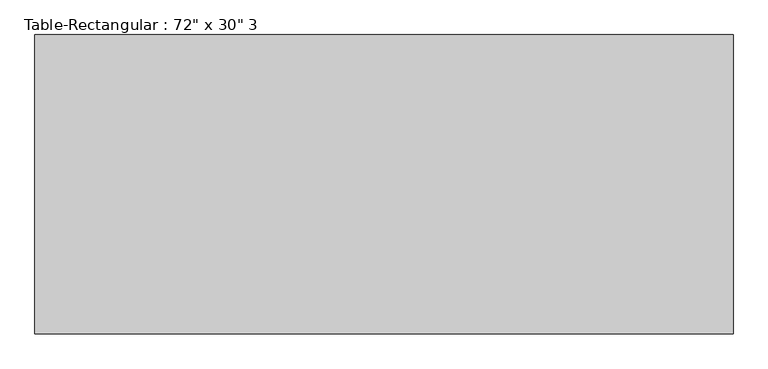
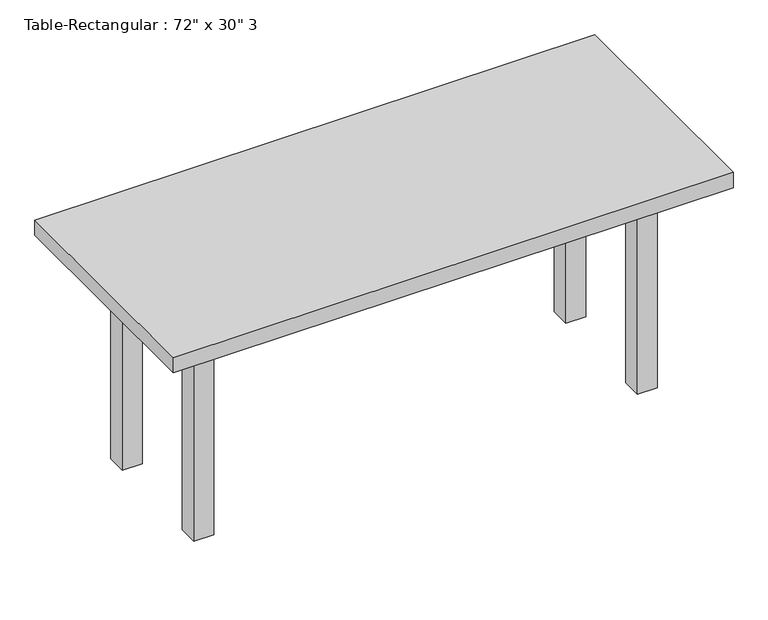
"""IFC4 building model written with IfcOpenShell, lengths in millimetres: furniture geometry."""

from ifc_helpers import new_model, si_unit, frame, origin, origin_with_axes, place, context, project, spatial, polyline, outline, extrude, source, transform, mapped, element, save


def furniture_102a29e2(model_context):
    return source(origin(), model_context, "Body", "SweptSolid", [
        extrude(outline(polyline([(-673.1, 228.6), (-673.1, 165.1), (-736.6, 165.1), (-736.6, 228.6), (-673.1, 228.6)])), origin_with_axes(), (0.0, 0.0, 1.0), 711.2),
        extrude(outline(polyline([(673.1, 228.6), (736.6, 228.6), (736.6, 165.1), (673.1, 165.1), (673.1, 228.6)])), origin_with_axes(), (0.0, 0.0, 1.0), 711.2),
        extrude(outline(polyline([(-673.1, -228.6), (-736.6, -228.6), (-736.6, -165.1), (-673.1, -165.1), (-673.1, -228.6)])), origin_with_axes(), (0.0, 0.0, 1.0), 711.2),
        extrude(outline(polyline([(673.1, -228.6), (673.1, -165.1), (736.6, -165.1), (736.6, -228.6), (673.1, -228.6)])), origin_with_axes(), (0.0, 0.0, 1.0), 711.2),
        extrude(outline(polyline([(889.0, 381.0), (889.0, -381.0), (-889.0, -381.0), (-889.0, 381.0), (889.0, 381.0)])), frame((0.0, 0.0, 711.2), z_axis=(0.0, 0.0, 1.0), x_axis=(1.0, 0.0, 0.0)), (0.0, 0.0, 1.0), 50.8),
        extrude(outline(polyline([(673.1, 190.5), (673.1, 165.1), (-673.1, 165.1), (-673.1, 190.5), (673.1, 190.5)])), frame((0.0, 0.0, 609.6), z_axis=(0.0, 0.0, 1.0), x_axis=(1.0, 0.0, 0.0)), (0.0, 0.0, 1.0), 101.6),
        extrude(outline(polyline([(673.1, -190.5), (-673.1, -190.5), (-673.1, -165.1), (673.1, -165.1), (673.1, -190.5)])), frame((0.0, 0.0, 609.6), z_axis=(0.0, 0.0, 1.0), x_axis=(1.0, 0.0, 0.0)), (0.0, 0.0, 1.0), 101.6),
        extrude(outline(polyline([(-685.8, -165.1), (-711.2, -165.1), (-711.2, 165.1), (-685.8, 165.1), (-685.8, -165.1)])), frame((0.0, 0.0, 609.6), z_axis=(0.0, 0.0, 1.0), x_axis=(1.0, 0.0, 0.0)), (0.0, 0.0, 1.0), 101.6),
        extrude(outline(polyline([(685.8, -165.1), (685.8, 165.1), (711.2, 165.1), (711.2, -165.1), (685.8, -165.1)])), frame((0.0, 0.0, 609.6), z_axis=(0.0, 0.0, 1.0), x_axis=(1.0, 0.0, 0.0)), (0.0, 0.0, 1.0), 101.6),
    ])


if __name__ == "__main__":
    model = new_model("IFC4")
    model_context = context("Model", 3, world=origin())
    ifc_project = project(units=[si_unit("LENGTHUNIT", "METRE", prefix="MILLI")], contexts=[model_context])
    site = spatial("IfcSite", under=ifc_project)
    building = spatial("IfcBuilding", under=site)
    placement = place(None, origin())
    furniture_shape = furniture_102a29e2(model_context)
    element("IfcFurniture", 1, ObjectType="Table-Rectangular : 72\" x 30\" 3", at=placement, inside=building, context=model_context, shape_type="MappedRepresentation", body=[
        mapped(furniture_shape, transform((0.0, 0.0, 0.0), x_axis=(1.0, 0.0, 0.0), y_axis=(0.0, 1.0, 0.0), z_axis=(0.0, 0.0, 1.0))),
    ])
    save(model, "model.ifc")

# Revit data of these elements
# Type "Table-Rectangular : 72\" x 30\" 3"
#   Assembly Code = "E2020200"
#   Height = 2' - 6"
#   Length = 5' - 10"
#   Width = 2' - 6"
#   Base Material = Birch
#   Top Material = Birch
#   Default Elevation = 0
# Element 1 (IfcFurniture, "Table-Rectangular : 72\" x 30\" 3")
#   Materials on its faces: "Birch"
# Materials
#   "Birch": class "Wood", colour RGB 224 178 126, transparency 0, Description = "Betula Alleghaniensis", Cost = 0
